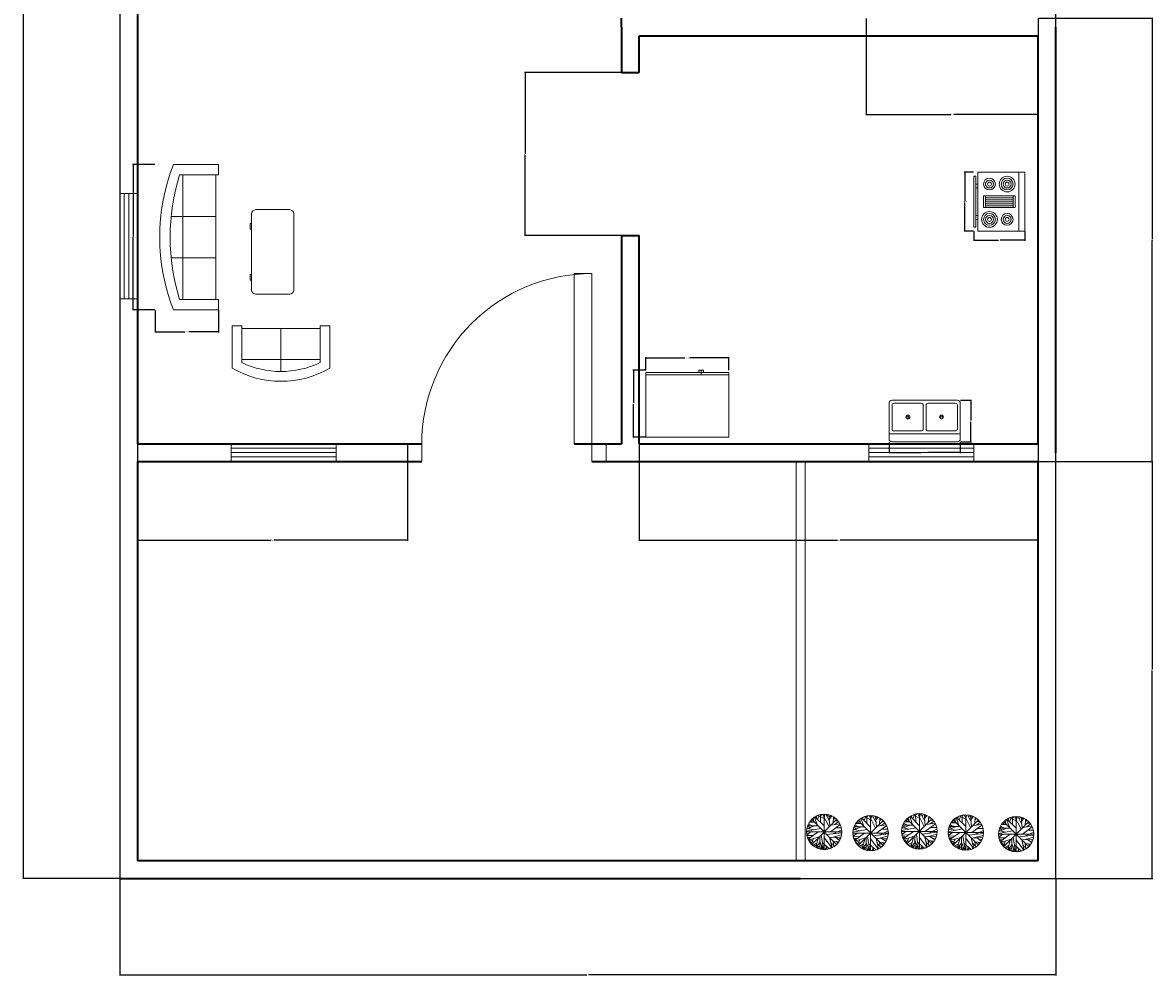
# Model space of a CAD drawing. Units: feet. Extents: x 2306 to 3052, y 829 to 1424.
# Tile 1 of 5: x 2306 to 2625, y 829 to 1098. Entities that reach past the tile are written whole.
import ezdxf

# ---------------------------------------------------------------- set-up
doc = ezdxf.new("R2010")
doc.units = ezdxf.units.FT
for name, color, linetype, lineweight in [('A-ANNO-DIMS', 2, 'Continuous', 18), ('A-DOOR', 3, 'Continuous', 18), ('A-EQPM', 9, 'Continuous', 18), ('A-FLOR-FIXT', 9, 'Continuous', 18), ('A-FLOR-OTLN', 7, 'Continuous', 25), ('A-FURN', 8, 'Continuous', 13), ('A-GLAZ', 4, 'Continuous', 18), ('A-WALL', 7, 'Continuous', 35), ('L-PLNT', 94, 'Continuous', 13)]:
    doc.layers.add(name, color=color, linetype=linetype, lineweight=lineweight)
doc.styles.get("Standard").update_dxf_attribs({"font": 'arial.ttf'})
doc.dimstyles.get("Standard").update_dxf_attribs({"dimtxt": 0.18, "dimasz": 0.18, "dimexe": 0.18, "dimexo": 0.0625, "dimgap": 0.09, "dimtad": 0, "dimtih": 1, "dimtoh": 1, "dimdec": 4, "dimzin": 0, "dimdsep": 46, "dimlunit": 4, "dimtxsty": 'Standard', "dimcen": 0.09, "dimadec": 0, "dimazin": 0, "dimtfac": 1, "dimtdec": 4, "dimtofl": 0, "dimtmove": 0, "dimatfit": 3, "dimfxl": 1, "dimtolj": 1, "dimtzin": 0, "dimarcsym": 0})

# ---------------------------------------------------------------- blocks, each defined once
blk = doc.blocks.new('Window - Wood Frame 36 in. Wide plan')
for p, q in [((0, 6), (0, 0)), ((0, 4.5), (36, 4.5)), ((36, 6), (36, 0)), ((0, 3), (36, 3)), ((0, 1.5), (36, 1.5))]:
    blk.add_line(p, q)
blk = doc.blocks.new('Sofa - Roundback 7 ft.')
for p, q in [((-36.000027, -34), (-36.000027, -11.4696)), ((-12.00002, -32.4421), (-12.00003, -6.5971)), ((11.99997, -32.4421), (11.99998, -6.5971)), ((35.99998, -34), (35.99998, -11.4696)), ((-35.999844, -13.3819), (35.9998, -13.3819)), ((-36.000027, -32.4421), (35.99998, -32.4421))]:
    blk.add_line(p, q)
for points in [[(-36.000027, -34), (-42.000027, -34), (-42.000027, -8)], [(41.99998, -8), (41.99998, -34), (35.99998, -34)]]:
    blk.add_lwpolyline(points)
for centre, radius, start, end in [((0, -114.25), 114.25, 68.43141, 111.5686), ((-0.00001, -127.1968), 121.1968, 72.72033, 107.2797)]:
    blk.add_arc(centre, radius, start, end)
blk = doc.blocks.new('Sofa - Roundback Loveseat 5 ft.')
for p, q in [((0, -32.44198), (0, -5.99998)), ((-24, -33.99998), (-24, -11.46958)), ((-23.9998, -13.38178), (23.99986, -13.38178)), ((24.00004, -33.99998), (24.00004, -11.46958)), ((-24, -32.44198), (24.00004, -32.44198))]:
    blk.add_line(p, q)
for points in [[(-24, -33.99998), (-30, -33.99998), (-30, -7.99998)], [(30.00004, -7.99998), (30.00004, -33.99998), (24.00004, -33.99998)]]:
    blk.add_lwpolyline(points)
for centre, radius, start, end in [((0, -60.24998), 60.24998, 60.13715, 119.8628), ((0, -61.38438), 55.38444, 64.32083, 115.6792)]:
    blk.add_arc(centre, radius, start, end)
blk = doc.blocks.new('Desk - 30 x 60 in.')
for p, q in [((-26.999995, 0), (26.999995, 0)), ((-29.999995, -27), (-29.999995, -3)), ((29.999995, -3), (29.999995, -27)), ((26.999995, -30), (-26.999995, -30)), ((-20.000005, -30), (-20.000005, -31)), ((-20.000005, -31), (-16.000005, -31)), ((-16.000005, -31), (-16.000005, -30)), ((15.999995, -31), (15.999995, -30)), ((19.999995, -31), (15.999995, -31)), ((19.999995, -30), (19.999995, -31))]:
    blk.add_line(p, q)
for centre, start, end in [((-26.499995, -3.5), 98.1301, 171.8699), ((26.499995, -3.5), 8.130102, 81.8699), ((-26.499995, -26.5), 188.1301, 261.8699), ((26.499995, -26.5), 278.1301, 351.8699)]:
    blk.add_arc(centre, 3.535534, start, end)
blk = doc.blocks.new('Range-Oven - 30 in top')
for p, q in [((0, -3), (30, -3)), ((12, -6), (18, -6)), ((13, -20), (13, -6)), ((14, -6), (14, -20)), ((15, -20), (15, -6)), ((16, -6), (16, -20)), ((17, -20), (17, -6)), ((18, -20), (12, -20)), ((6, -24), (6, -25)), ((8, -25), (8, -24)), ((22, -25), (22, -24)), ((24, -24), (24, -25))]:
    blk.add_line(p, q)
for points in [[(0, -24), (0, 0), (30, 0), (30, -24)], [(12, -21), (12, -5), (18, -5), (18, -21)], [(2, -26), (2, -25), (28, -25), (28, -26)]]:
    blk.add_lwpolyline(points, close=True)
for centre, radius in [((6, -9), 4), ((6, -9), 3), ((6, -9), 2), ((6, -9), 1), ((24, -9), 3), ((24, -9), 2), ((24, -9), 1), ((6, -18), 3), ((6, -18), 2), ((6, -18), 1), ((24, -18), 4), ((24, -18), 3), ((24, -18), 2), ((24, -18), 1)]:
    blk.add_circle(centre, radius)
blk = doc.blocks.new('Sink-double - 36 in top')
for p, q in [((-18, -4), (18, -4)), ((-0.75, -18.5), (-0.75, -6.5)), ((0.75, -6.5), (0.75, -18.5))]:
    blk.add_line(p, q)
for points in [[(-16.5, 0), (16.5, 0)], [(-18, -19.5), (-18, -1.5)], [(-15.5, -5.5), (-1.75, -5.5)], [(1.75, -5.5), (15.5, -5.5)], [(18, -1.5), (18, -19.5)], [(-16.5, -18.5), (-16.5, -6.5)], [(16.5, -6.5), (16.5, -18.5)], [(16.5, -21), (-16.5, -21)], [(-1.75, -19.5), (-15.5, -19.5)], [(15.5, -19.5), (1.75, -19.5)]]:
    blk.add_lwpolyline(points)
for centre, radius in [((-8.5, -12.5), 1), ((-8.5, -12.5), 0.5), ((8.5, -12.5), 1), ((8.5, -12.5), 0.5)]:
    blk.add_circle(centre, radius)
for centre, radius, start, end in [((-16.5, -1.5), 1.5, 90, 180), ((16.5, -1.5), 1.5, 0, 90), ((-15.5, -6.5), 1, 90, 180), ((-1.75, -6.5), 1, 0, 90), ((1.75, -6.5), 1, 90, 180), ((15.5, -6.5), 1, 0, 90), ((-16.5, -19.5), 1.5, 180, 270), ((-15.5, -18.5), 1, 180, 270), ((-1.75, -18.5), 1, 270, 0), ((1.75, -18.5), 1, 180, 270), ((15.5, -18.5), 1, 270, 0), ((16.5, -19.5), 1.5, 270, 0)]:
    blk.add_arc(centre, radius, start, end)
blk = doc.blocks.new('Refrigerator-2 door - 36 in top')
for p, q in [((0, -26.999999), (36, -26.999999)), ((11, -27.999999), (11, -28.999999)), ((11, -28.999999), (13, -28.999999)), ((12, -26.999999), (12, -28.999999)), ((13, -28.999999), (13, -27.999999))]:
    blk.add_line(p, q)
blk.add_lwpolyline([(0, -27.999999), (0, 0), (36, 0), (36, -27.999999)], close=True)
blk = doc.blocks.new('Tree - deciduous plan')
for p, q in [((-43.8768, 36.4326), (-44.405, 40.2696)), ((42, 42), (-42, -42)), ((42, -42), (-42, 42)), ((-40.1797, 44.558), (-36.4825, 43.2038)), ((-37.0107, 47.0408), (-35.25, 35.5298)), ((-32.6092, 50.4264), (-23.2782, 23.5674)), ((-31.2008, 51.1035), (-0.2149, 20.1818)), ((-26.4472, 46.5894), (-26.2712, 53.8116)), ((-22.0458, 42.0753), (-16.5881, 57.6486)), ((-21.1656, 55.8436), (-0.0388, 45.0094)), ((-12.5388, 54.9406), (-7.9613, 59.4546)), ((-12.3627, 32.1443), (-12.5388, 58.7776)), ((-5.3205, 59.6806), (16.5105, 16.7963)), ((2.426, 54.9406), (-1.4472, 59.9056)), ((0, 59.9996), (0, -60)), ((0.4894, 48.6208), (3.6584, 59.6806)), ((18.2711, 35.5298), (5.419, 59.6806)), ((9.8203, 51.5549), (12.8133, 58.5516)), ((19.6795, 19.5047), (16.3344, 57.6486)), ((17.0387, 51.1035), (23.2006, 55.1666)), ((17.7429, 43.6552), (25.4894, 54.2636)), ((31.6513, 50.8778), (30.2429, 30.5643)), ((31.1232, 42.5267), (35.8767, 48.1693)), ((-59.7219, 2.8025), (-12.0106, 12.0565)), ((-32.2571, 20.6333), (-59.1937, 9.348)), ((-58.6656, 12.7336), (-35.9543, 7.5424)), ((-57.081, 17.9248), (-47.0458, 14.7649)), ((-56.0247, 20.859), (-20.8134, 20.859)), ((-54.7923, 24.4702), (-47.75, 21.0847)), ((-54.6162, -24.7335), (-20.2853, 0.0941)), ((-53.2078, 27.4044), (-40.1797, 20.859)), ((-49.8627, 32.8214), (-32.7853, 32.8214)), ((-45.8134, 38.2383), (-40.5318, 33.0471)), ((54.3626, 25.3731), (20.9119, 0.3198)), ((23.3767, 23.3417), (53.3063, 27.4044)), ((29.3626, -6.6771), (59.4682, 7.091)), ((36.2288, 25.1474), (48.9049, 35.0784)), ((37.1091, 37.1098), (46.6161, 37.5612)), ((38.5175, 13.4107), (58.2359, 13.6364)), ((-60, 0), (60, 0)), ((-59.7219, -4.8714), (-54.2641, -6.6771)), ((-45.2853, -0.1316), (-59.0177, -10.0627)), ((-58.4895, -12.3197), (-36.4825, -11.6426)), ((-57.081, -18.4138), (-45.2853, -17.9624)), ((-52.6797, -18.188), (-55.4966, -22.0251)), ((-53.2078, -27.442), (-16.7641, -16.6081)), ((-38.9472, -29.0219), (-51.4472, -30.6018)), ((-47.2219, -19.3166), (-50.2148, -26.3135)), ((-46.5177, -30.1504), (-49.5106, -33.536)), ((-32.4331, -32.4075), (-48.1021, -35.5674)), ((-43.7008, -34.6645), (-46.6937, -37.373)), ((-35.9543, -22.4765), (-44.0529, -40.5329)), ((-24.6867, -37.8244), (-38.7712, -45.7241)), ((-19.9331, -20.2194), (-28.5599, -52.721)), ((-14.6515, -36.2445), (-27.6797, -52.9467)), ((-14.8275, -15.0282), (-14.6515, -57.6865)), ((-14.6515, -32.1818), (-3.912, -59.4922)), ((-10.074, -10.0627), (-2.5036, -59.7178)), ((-6.2008, -36.2445), (17.919, -57.0094)), ((-0.0388, -19.0909), (25.8415, -53.8495)), ((9.2922, -9.1598), (59.6443, -2.8401)), ((18.6232, -18.6394), (26.7218, -53.3981)), ((18.7992, -18.6394), (57.3556, -17.2853)), ((22.8485, -36.4702), (35.3485, -48.4326)), ((26.3697, -18.4138), (58.9401, -9.8369)), ((30.419, -30.1504), (32.3556, -50.0125)), ((31.4753, -31.279), (49.6091, -33.3103)), ((38.1654, -18.188), (52.426, -29.0219)), ((41.5105, -32.6332), (46.088, -38.0501)), ((45.9119, -24.0564), (55.595, -22.2508)), ((-26.2712, -43.9185), (-34.7219, -48.6583)), ((-14.6515, -47.3041), (-25.0388, -54.3009)), ((-21.5177, -45.4984), (-19.9331, -56.1065)), ((-8.4895, -47.5298), (-11.4825, -58.5893)), ((-6.3768, -52.721), (-9.3698, -58.815)), ((8.4119, -53.1724), (3.8344, -59.4922)), ((5.9471, -46.6269), (10.5246, -58.5893)), ((24.7852, -44.8213), (23.0246, -54.978))]:
    blk.add_line(p, q)
blk.add_circle((0, 0), 60)
blk = doc.blocks.new('DOOR-SWING-WIDE')
blk.add_lwpolyline([(52, 53), (52, 5), (56, 5), (56, 0), (52, 0), (52, 5), (47, 5), (47, 53), (48, 53), (52, 53, 0.414214), (4, 5)], format="xyb")
blk.add_lwpolyline([(4, 5), (4, 0), (0, 0), (0, 5)], close=True)
blk = doc.blocks.new('*D32')
at = {"layer": 'A-ANNO-DIMS', "color": 0, "lineweight": -2, "transparency": 16777216}
for p, q in [((2343.71, 1058.11), (2337.44, 1058.11)), ((2337.62, 1057.93), (2337.62, 1037.77)), ((2337.62, 1017.24), (2337.62, 1037.41)), ((2343.71, 1017.06), (2337.44, 1017.06))]:
    blk.add_line(p, q, dxfattribs=at)
at = {"layer": 'A-ANNO-DIMS', "color": 0, "transparency": 16777216}
for points in [[(2337.59, 1057.93), (2337.65, 1057.93), (2337.62, 1058.11)], [(2337.59, 1017.24), (2337.65, 1017.24), (2337.62, 1017.06)]]:
    blk.add_solid(points, dxfattribs=at)
at = {"layer": 'Defpoints', "color": 0, "transparency": 16777216}
for p in [(2337.62, 1058.11), (2343.77, 1058.11), (2343.77, 1017.06)]:
    blk.add_point(p, dxfattribs=at)
at = {"layer": 'A-ANNO-DIMS', "color": 0, "transparency": 16777216, "insert": (2337.62, 1037.59), "char_height": 0.18, "attachment_point": 5}
blk.add_mtext('\\A1;SOFA 41 TYP.', dxfattribs=at)
blk = doc.blocks.new('*D33')
at = {"layer": 'A-ANNO-DIMS', "color": 0, "lineweight": -2, "transparency": 16777216}
for p, q in [((2343.77, 1017), (2343.77, 1010.73)), ((2361.69, 1017), (2361.69, 1010.73)), ((2343.95, 1010.91), (2352.21, 1010.91)), ((2361.51, 1010.91), (2353.25, 1010.91))]:
    blk.add_line(p, q, dxfattribs=at)
at = {"layer": 'A-ANNO-DIMS', "color": 0, "transparency": 16777216}
for points in [[(2343.95, 1010.94), (2343.95, 1010.88), (2343.77, 1010.91)], [(2361.51, 1010.94), (2361.51, 1010.88), (2361.69, 1010.91)]]:
    blk.add_solid(points, dxfattribs=at)
at = {"layer": 'Defpoints', "color": 0, "transparency": 16777216}
for p in [(2343.77, 1017.06), (2361.69, 1017.06), (2343.77, 1010.91)]:
    blk.add_point(p, dxfattribs=at)
at = {"layer": 'A-ANNO-DIMS', "color": 0, "transparency": 16777216, "insert": (2352.73, 1010.91), "char_height": 0.18, "attachment_point": 5}
blk.add_mtext('\\A1;18 TYP.', dxfattribs=at)
blk = doc.blocks.new('*D40')
at = {"layer": 'A-ANNO-DIMS', "color": 0, "lineweight": -2, "transparency": 16777216}
for p, q in [((2574.57, 1055.88), (2571.96, 1055.88)), ((2572.14, 1055.7), (2572.14, 1047.76)), ((2572.14, 1039.45), (2572.14, 1047.39)), ((2574.57, 1039.27), (2571.96, 1039.27))]:
    blk.add_line(p, q, dxfattribs=at)
at = {"layer": 'A-ANNO-DIMS', "color": 0, "transparency": 16777216}
for points in [[(2572.11, 1055.7), (2572.17, 1055.7), (2572.14, 1055.88)], [(2572.11, 1039.45), (2572.17, 1039.45), (2572.14, 1039.27)]]:
    blk.add_solid(points, dxfattribs=at)
at = {"layer": 'Defpoints', "color": 0, "transparency": 16777216}
for p in [(2574.64, 1055.88), (2572.14, 1039.27), (2574.64, 1039.27)]:
    blk.add_point(p, dxfattribs=at)
at = {"layer": 'A-ANNO-DIMS', "color": 0, "transparency": 16777216, "insert": (2572.14, 1047.58), "char_height": 0.18, "attachment_point": 5}
blk.add_mtext('\\A1;RANGE 17', dxfattribs=at)
blk = doc.blocks.new('*D41')
at = {"layer": 'A-ANNO-DIMS', "color": 0, "lineweight": -2, "transparency": 16777216}
for p, q in [((2574.64, 1039.21), (2574.64, 1036.6)), ((2574.82, 1036.78), (2581.63, 1036.78)), ((2588.86, 1036.78), (2582.05, 1036.78)), ((2589.04, 1039.21), (2589.04, 1036.6))]:
    blk.add_line(p, q, dxfattribs=at)
at = {"layer": 'A-ANNO-DIMS', "color": 0, "transparency": 16777216}
for points in [[(2574.82, 1036.81), (2574.82, 1036.75), (2574.64, 1036.78)], [(2588.86, 1036.81), (2588.86, 1036.75), (2589.04, 1036.78)]]:
    blk.add_solid(points, dxfattribs=at)
at = {"layer": 'Defpoints', "color": 0, "transparency": 16777216}
for p in [(2574.64, 1039.27), (2589.04, 1039.27), (2589.04, 1036.78)]:
    blk.add_point(p, dxfattribs=at)
at = {"layer": 'A-ANNO-DIMS', "color": 0, "transparency": 16777216, "insert": (2581.84, 1036.78), "char_height": 0.18, "attachment_point": 5}
blk.add_mtext('\\A1;14', dxfattribs=at)
blk = doc.blocks.new('*D42')
at = {"layer": 'A-ANNO-DIMS', "color": 0, "lineweight": -2, "transparency": 16777216}
for p, q in [((2550.75, 979.83), (2550.75, 976.7)), ((2570.84, 979.83), (2570.84, 976.7)), ((2550.93, 976.88), (2559.7, 976.88)), ((2570.66, 976.88), (2561.89, 976.88))]:
    blk.add_line(p, q, dxfattribs=at)
at = {"layer": 'A-ANNO-DIMS', "color": 0, "transparency": 16777216}
for points in [[(2550.93, 976.91), (2550.93, 976.85), (2550.75, 976.88)], [(2570.66, 976.91), (2570.66, 976.85), (2570.84, 976.88)]]:
    blk.add_solid(points, dxfattribs=at)
at = {"layer": 'Defpoints', "color": 0, "transparency": 16777216}
for p in [(2550.75, 979.89), (2570.84, 979.89), (2550.75, 976.88)]:
    blk.add_point(p, dxfattribs=at)
at = {"layer": 'A-ANNO-DIMS', "color": 0, "transparency": 16777216, "insert": (2560.79, 976.88), "char_height": 0.18, "attachment_point": 5}
blk.add_mtext('\\A1;DOUBLE SINK 20', dxfattribs=at)
blk = doc.blocks.new('*D43')
at = {"layer": 'A-ANNO-DIMS', "color": 0, "lineweight": -2, "transparency": 16777216}
for p, q in [((2570.9, 991.61), (2574.03, 991.61)), ((2573.85, 991.43), (2573.85, 985.93)), ((2573.85, 980.07), (2573.85, 985.57)), ((2570.9, 979.89), (2574.03, 979.89))]:
    blk.add_line(p, q, dxfattribs=at)
at = {"layer": 'A-ANNO-DIMS', "color": 0, "transparency": 16777216}
for points in [[(2573.82, 991.43), (2573.88, 991.43), (2573.85, 991.61)], [(2573.82, 980.07), (2573.88, 980.07), (2573.85, 979.89)]]:
    blk.add_solid(points, dxfattribs=at)
at = {"layer": 'Defpoints', "color": 0, "transparency": 16777216}
for p in [(2570.84, 991.61), (2570.84, 979.89), (2573.85, 979.89)]:
    blk.add_point(p, dxfattribs=at)
at = {"layer": 'A-ANNO-DIMS', "color": 0, "transparency": 16777216, "insert": (2573.85, 985.75), "char_height": 0.18, "attachment_point": 5}
blk.add_mtext('\\A1;12', dxfattribs=at)
blk = doc.blocks.new('*D44')
at = {"layer": 'A-ANNO-DIMS', "color": 0, "lineweight": -2, "transparency": 16777216}
for p, q in [((2482.2, 1000.12), (2482.2, 1003.74)), ((2482.38, 1003.56), (2493.15, 1003.56)), ((2505.37, 1003.56), (2494.6, 1003.56)), ((2505.55, 1000.12), (2505.55, 1003.74))]:
    blk.add_line(p, q, dxfattribs=at)
at = {"layer": 'A-ANNO-DIMS', "color": 0, "transparency": 16777216}
for points in [[(2482.38, 1003.59), (2482.38, 1003.53), (2482.2, 1003.56)], [(2505.37, 1003.59), (2505.37, 1003.53), (2505.55, 1003.56)]]:
    blk.add_solid(points, dxfattribs=at)
at = {"layer": 'Defpoints', "color": 0, "transparency": 16777216}
for p in [(2482.2, 1003.56), (2482.2, 1000.06), (2505.55, 1000.06)]:
    blk.add_point(p, dxfattribs=at)
at = {"layer": 'A-ANNO-DIMS', "color": 0, "transparency": 16777216, "insert": (2493.87, 1003.56), "char_height": 0.18, "attachment_point": 5}
blk.add_mtext('\\A1;FRIDGE 23', dxfattribs=at)
blk = doc.blocks.new('*D45')
at = {"layer": 'A-ANNO-DIMS', "color": 0, "lineweight": -2, "transparency": 16777216}
for p, q in [((2482.13, 1000.06), (2478.51, 1000.06)), ((2478.69, 999.88), (2478.69, 990.84)), ((2478.69, 981.43), (2478.69, 990.48)), ((2482.13, 981.25), (2478.51, 981.25))]:
    blk.add_line(p, q, dxfattribs=at)
at = {"layer": 'A-ANNO-DIMS', "color": 0, "transparency": 16777216}
for points in [[(2478.66, 999.88), (2478.72, 999.88), (2478.69, 1000.06)], [(2478.66, 981.43), (2478.72, 981.43), (2478.69, 981.25)]]:
    blk.add_solid(points, dxfattribs=at)
at = {"layer": 'Defpoints', "color": 0, "transparency": 16777216}
for p in [(2482.2, 1000.06), (2478.69, 981.25), (2482.2, 981.25)]:
    blk.add_point(p, dxfattribs=at)
at = {"layer": 'A-ANNO-DIMS', "color": 0, "transparency": 16777216, "insert": (2478.69, 990.66), "char_height": 0.18, "attachment_point": 5}
blk.add_mtext('\\A1;19', dxfattribs=at)
blk = doc.blocks.new('*D46')
at = {"layer": 'A-ANNO-DIMS', "color": 0, "lineweight": -2, "transparency": 16777216}
for p, q in [((2333.8, 856.76), (2333.8, 829.47)), ((2597.8, 856.76), (2597.8, 829.47)), ((2333.98, 829.65), (2465.51, 829.65)), ((2597.62, 829.65), (2466.09, 829.65))]:
    blk.add_line(p, q, dxfattribs=at)
at = {"layer": 'A-ANNO-DIMS', "color": 0, "transparency": 16777216}
for points in [[(2333.98, 829.68), (2333.98, 829.62), (2333.8, 829.65)], [(2597.62, 829.68), (2597.62, 829.62), (2597.8, 829.65)]]:
    blk.add_solid(points, dxfattribs=at)
at = {"layer": 'Defpoints', "color": 0, "transparency": 16777216}
for p in [(2333.8, 856.83), (2597.8, 856.83), (2597.8, 829.65)]:
    blk.add_point(p, dxfattribs=at)
at = {"layer": 'A-ANNO-DIMS', "color": 0, "transparency": 16777216, "insert": (2465.8, 829.65), "char_height": 0.18, "attachment_point": 5}
blk.add_mtext('\\A1;264', dxfattribs=at)
blk = doc.blocks.new('*D47')
at = {"layer": 'A-ANNO-DIMS', "color": 0, "lineweight": -2, "transparency": 16777216}
for p, q in [((2333.74, 1396.83), (2306.45, 1396.83)), ((2306.63, 1396.65), (2306.63, 1127.01)), ((2306.63, 857.01), (2306.63, 1126.65)), ((2333.74, 856.83), (2306.45, 856.83))]:
    blk.add_line(p, q, dxfattribs=at)
at = {"layer": 'A-ANNO-DIMS', "color": 0, "transparency": 16777216}
for points in [[(2306.6, 1396.65), (2306.66, 1396.65), (2306.63, 1396.83)], [(2306.6, 857.01), (2306.66, 857.01), (2306.63, 856.83)]]:
    blk.add_solid(points, dxfattribs=at)
at = {"layer": 'Defpoints', "color": 0, "transparency": 16777216}
for p in [(2306.63, 1396.83), (2333.8, 1396.83), (2333.8, 856.83)]:
    blk.add_point(p, dxfattribs=at)
at = {"layer": 'A-ANNO-DIMS', "color": 0, "transparency": 16777216, "insert": (2306.63, 1126.83), "char_height": 0.18, "attachment_point": 5}
blk.add_mtext('\\A1;540', dxfattribs=at)
blk = doc.blocks.new('*D48')
at = {"layer": 'A-ANNO-DIMS', "color": 0, "lineweight": -2, "transparency": 16777216}
for p, q in [((2592.87, 974.33), (2625.16, 974.33)), ((2624.98, 974.15), (2624.98, 915.76)), ((2624.98, 857.01), (2624.98, 915.4)), ((2597.87, 856.83), (2625.16, 856.83))]:
    blk.add_line(p, q, dxfattribs=at)
at = {"layer": 'A-ANNO-DIMS', "color": 0, "transparency": 16777216}
for points in [[(2624.95, 974.15), (2625.01, 974.15), (2624.98, 974.33)], [(2624.95, 857.01), (2625.01, 857.01), (2624.98, 856.83)]]:
    blk.add_solid(points, dxfattribs=at)
at = {"layer": 'Defpoints', "color": 0, "transparency": 16777216}
for p in [(2592.8, 974.33), (2624.98, 974.33), (2597.8, 856.83)]:
    blk.add_point(p, dxfattribs=at)
at = {"layer": 'A-ANNO-DIMS', "color": 0, "transparency": 16777216, "insert": (2624.98, 915.58), "char_height": 0.18, "attachment_point": 5}
blk.add_mtext('\\A1;117.5', dxfattribs=at)
blk = doc.blocks.new('*D49')
at = {"layer": 'A-ANNO-DIMS', "color": 0, "lineweight": -2, "transparency": 16777216}
for p, q in [((2592.87, 1099.33), (2625.16, 1099.33)), ((2624.98, 1099.15), (2624.98, 1037.01)), ((2624.98, 974.51), (2624.98, 1036.65)), ((2592.87, 974.33), (2625.16, 974.33))]:
    blk.add_line(p, q, dxfattribs=at)
at = {"layer": 'A-ANNO-DIMS', "color": 0, "transparency": 16777216}
for points in [[(2624.95, 1099.15), (2625.01, 1099.15), (2624.98, 1099.33)], [(2624.95, 974.51), (2625.01, 974.51), (2624.98, 974.33)]]:
    blk.add_solid(points, dxfattribs=at)
at = {"layer": 'Defpoints', "color": 0, "transparency": 16777216}
for p in [(2592.8, 1099.33), (2624.98, 1099.33), (2592.8, 974.33)]:
    blk.add_point(p, dxfattribs=at)
at = {"layer": 'A-ANNO-DIMS', "color": 0, "transparency": 16777216, "insert": (2624.98, 1036.83), "char_height": 0.18, "attachment_point": 5}
blk.add_mtext('\\A1;125', dxfattribs=at)
blk = doc.blocks.new('*D57')
at = {"layer": 'A-ANNO-DIMS', "color": 0, "lineweight": -2, "transparency": 16777216}
for p, q in [((2480.3, 979.26), (2480.3, 951.97)), ((2592.8, 979.26), (2592.8, 951.97)), ((2480.48, 952.15), (2536.17, 952.15)), ((2592.62, 952.15), (2536.94, 952.15))]:
    blk.add_line(p, q, dxfattribs=at)
at = {"layer": 'A-ANNO-DIMS', "color": 0, "transparency": 16777216}
for points in [[(2480.48, 952.18), (2480.48, 952.12), (2480.3, 952.15)], [(2592.62, 952.18), (2592.62, 952.12), (2592.8, 952.15)]]:
    blk.add_solid(points, dxfattribs=at)
at = {"layer": 'Defpoints', "color": 0, "transparency": 16777216}
for p in [(2480.3, 979.33), (2592.8, 979.33), (2480.3, 952.15)]:
    blk.add_point(p, dxfattribs=at)
at = {"layer": 'A-ANNO-DIMS', "color": 0, "transparency": 16777216, "insert": (2536.55, 952.15), "char_height": 0.18, "attachment_point": 5}
blk.add_mtext('\\A1;112.5', dxfattribs=at)
blk = doc.blocks.new('*D58')
at = {"layer": 'A-ANNO-DIMS', "color": 0, "lineweight": -2, "transparency": 16777216}
for p, q in [((2338.8, 979.26), (2338.8, 951.97)), ((2414.97, 979.26), (2414.97, 951.97)), ((2338.98, 952.15), (2376.5, 952.15)), ((2414.79, 952.15), (2377.28, 952.15))]:
    blk.add_line(p, q, dxfattribs=at)
at = {"layer": 'A-ANNO-DIMS', "color": 0, "transparency": 16777216}
for points in [[(2338.98, 952.18), (2338.98, 952.12), (2338.8, 952.15)], [(2414.79, 952.18), (2414.79, 952.12), (2414.97, 952.15)]]:
    blk.add_solid(points, dxfattribs=at)
at = {"layer": 'Defpoints', "color": 0, "transparency": 16777216}
for p in [(2338.8, 979.33), (2414.97, 979.33), (2338.8, 952.15)]:
    blk.add_point(p, dxfattribs=at)
at = {"layer": 'A-ANNO-DIMS', "color": 0, "transparency": 16777216, "insert": (2376.89, 952.15), "char_height": 0.18, "attachment_point": 5}
blk.add_mtext('\\A1;76.17', dxfattribs=at)
blk = doc.blocks.new('*D60')
at = {"layer": 'A-ANNO-DIMS', "color": 0, "lineweight": -2, "transparency": 16777216}
for p, q in [((2475.24, 1083.97), (2447.95, 1083.97)), ((2448.13, 1083.79), (2448.13, 1061.21)), ((2448.13, 1038.26), (2448.13, 1060.84)), ((2475.24, 1038.08), (2447.95, 1038.08))]:
    blk.add_line(p, q, dxfattribs=at)
at = {"layer": 'A-ANNO-DIMS', "color": 0, "transparency": 16777216}
for points in [[(2448.1, 1083.79), (2448.16, 1083.79), (2448.13, 1083.97)], [(2448.1, 1038.26), (2448.16, 1038.26), (2448.13, 1038.08)]]:
    blk.add_solid(points, dxfattribs=at)
at = {"layer": 'Defpoints', "color": 0, "transparency": 16777216}
for p in [(2448.13, 1083.97), (2475.3, 1083.97), (2475.3, 1038.08)]:
    blk.add_point(p, dxfattribs=at)
at = {"layer": 'A-ANNO-DIMS', "color": 0, "transparency": 16777216, "insert": (2448.13, 1061.02), "char_height": 0.18, "attachment_point": 5}
blk.add_mtext('\\A1;45.89', dxfattribs=at)
blk = doc.blocks.new('*D61')
at = {"layer": 'A-ANNO-DIMS', "color": 0, "lineweight": -2, "transparency": 16777216}
for p, q in [((2544.34, 1099.26), (2544.34, 1071.97)), ((2592.8, 1099.26), (2592.8, 1071.97)), ((2544.52, 1072.15), (2568.17, 1072.15)), ((2592.62, 1072.15), (2568.97, 1072.15))]:
    blk.add_line(p, q, dxfattribs=at)
at = {"layer": 'A-ANNO-DIMS', "color": 0, "transparency": 16777216}
for points in [[(2544.52, 1072.18), (2544.52, 1072.12), (2544.34, 1072.15)], [(2592.62, 1072.18), (2592.62, 1072.12), (2592.8, 1072.15)]]:
    blk.add_solid(points, dxfattribs=at)
at = {"layer": 'Defpoints', "color": 0, "transparency": 16777216}
for p in [(2544.34, 1099.33), (2592.8, 1099.33), (2544.34, 1072.15)]:
    blk.add_point(p, dxfattribs=at)
at = {"layer": 'A-ANNO-DIMS', "color": 0, "transparency": 16777216, "insert": (2568.57, 1072.15), "char_height": 0.18, "attachment_point": 5}
blk.add_mtext('\\A1;48.47', dxfattribs=at)

msp = doc.modelspace()

# ---------------------------------------------------------------- linework, layer by layer
at = {"layer": 'A-FLOR-OTLN'}
for p, q in [((2333.803, 1396.827), (2333.803, 856.827)), ((2597.803, 856.827), (2597.803, 1396.827)), ((2333.803, 856.827), (2597.803, 856.827))]:
    msp.add_line(p, q, dxfattribs=at)
at = {"layer": 'A-WALL'}
for p, q in [((2338.803, 1250.327), (2338.803, 979.327)), ((2475.303, 1096.827), (2475.303, 1099.327)), ((2475.303, 1096.827), (2475.303, 1083.971)), ((2480.303, 1094.327), (2592.803, 1094.327)), ((2480.303, 1083.971), (2480.303, 1094.327)), ((2592.803, 979.327), (2592.803, 1094.327)), ((2597.803, 976.827), (2597.803, 1096.827)), ((2475.303, 1083.971), (2480.303, 1083.971)), ((2475.303, 1038.077), (2480.303, 1038.077)), ((2475.303, 1038.077), (2475.303, 979.327)), ((2480.303, 979.327), (2480.303, 1038.077)), ((2338.803, 979.327), (2418.974, 979.327)), ((2461.974, 979.327), (2475.303, 979.327)), ((2480.303, 979.327), (2501.803, 979.327)), ((2501.803, 979.327), (2592.803, 979.327)), ((2338.803, 974.327), (2418.974, 974.327)), ((2338.803, 974.327), (2338.803, 861.827)), ((2466.974, 974.327), (2501.803, 974.327)), ((2501.803, 974.327), (2592.803, 974.327)), ((2523.303, 974.327), (2525.803, 974.327)), ((2592.803, 861.827), (2592.803, 974.327)), ((2338.803, 861.827), (2592.803, 861.827)), ((2338.803, 861.827), (2525.803, 861.827)), ((2333.803, 856.827), (2525.803, 856.827))]:
    msp.add_line(p, q, dxfattribs=at)
at = {"layer": 'L-PLNT'}
for p, q in [((2524.553, 974.327), (2524.553, 861.827)), ((2524.553, 974.327), (2527.053, 974.327)), ((2527.053, 861.827), (2527.053, 974.327))]:
    msp.add_line(p, q, dxfattribs=at)

# ---------------------------------------------------------------- block references
at = {"layer": 'A-DOOR'}
msp.add_blockref('DOOR-SWING-WIDE', (2414.974, 974.327), dxfattribs=at)
at = {"layer": 'A-EQPM'}
for name, p, xscale, yscale, zscale, rotation in [('Range-Oven - 30 in top', (2589.035, 1055.884), 0.5538035962556707, 0.5538035962556707, 0.5538035962556707, 270), ('Refrigerator-2 door - 36 in top', (2505.547, 981.252), 0.6485986588828088, 0.6485986588828088, 0.6485986588828088, 180)]:
    msp.add_blockref(name, p, dxfattribs=dict(at, xscale=xscale, yscale=yscale, zscale=zscale, rotation=rotation))
at = {"layer": 'A-FLOR-FIXT', "xscale": 0.5580233951230867, "yscale": 0.5580233951230867, "zscale": 0.5580233951230867, "rotation": 180}
msp.add_blockref('Sink-double - 36 in top', (2560.794, 979.895), dxfattribs=at)
at = {"layer": 'A-FURN'}
for name, p, xscale, yscale, zscale, rotation in [('Sofa - Roundback 7 ft.', (2345.076, 1037.589), 0.4886678051459193, 0.4886678051459193, 0.4886678051459193, 90), ('Desk - 30 x 60 in.', (2382.902, 1033.44), 0.3981448877142051, 0.3981448877142051, 0.3981448877142051, 270), ('Sofa - Roundback Loveseat 5 ft.', (2379.267, 996.965), 0.4591894755531339, 0.4591894755531339, 0.4591894755531339, 180)]:
    msp.add_blockref(name, p, dxfattribs=dict(at, xscale=xscale, yscale=yscale, zscale=zscale, rotation=rotation))
at = {"layer": 'A-GLAZ', "xscale": 0.82338841385576, "yscale": 0.82338841385576, "zscale": 0.82338841385576, "rotation": 90}
msp.add_blockref('Window - Wood Frame 36 in. Wide plan', (2338.803, 1020.247), dxfattribs=at)
at = {"layer": 'A-GLAZ', "xscale": 0.82338841385576, "yscale": 0.82338841385576, "zscale": 0.82338841385576}
for p in [(2365.2, 974.387), (2545.006, 974.387)]:
    msp.add_blockref('Window - Wood Frame 36 in. Wide plan', p, dxfattribs=at)
at = {"layer": 'L-PLNT', "xscale": 0.0833333333333333, "yscale": 0.0833333333333333, "zscale": 0.0833333333333333}
for p in [(2532.448, 869.911), (2545.547, 869.592), (2559.286, 870.071), (2572.385, 869.751), (2586.605, 869.261)]:
    msp.add_blockref('Tree - deciduous plan', p, dxfattribs=at)

# ---------------------------------------------------------------- dimensions: what is measured, and where the dimension line sits
at = {"layer": 'A-ANNO-DIMS'}
for base, p1, p2, angle, override, picture, middle in [((2306.628, 1396.827), (2333.803, 856.827), (2333.803, 1396.827), 90, {"dimdec": 0, "dimlfac": 1, "dimrnd": 0, "dimzin": 0, "dimdsep": 46, "dimlunit": 2}, '*D47', (2306.628, 1126.827)), ((2544.336, 1072.152), (2592.803, 1099.327), (2544.336, 1099.327), 180, {"dimdec": 2, "dimlfac": 1, "dimrnd": 0, "dimzin": 0, "dimdsep": 46, "dimlunit": 2}, '*D61', (2568.57, 1072.152)), ((2624.978, 1099.327), (2592.803, 974.327), (2592.803, 1099.327), 90, {"dimdec": 0, "dimlfac": 1, "dimrnd": 0, "dimzin": 0, "dimdsep": 46, "dimlunit": 2}, '*D49', (2624.978, 1036.827)), ((2448.128, 1083.971), (2475.303, 1038.077), (2475.303, 1083.971), 90, {"dimdec": 2, "dimlfac": 1, "dimrnd": 0, "dimzin": 0, "dimdsep": 46, "dimlunit": 2}, '*D60', (2448.128, 1061.024)), ((2478.695, 981.252), (2482.197, 1000.062), (2482.197, 981.252), 270, {"dimdec": 0, "dimlfac": 1, "dimrnd": 0, "dimzin": 0, "dimdsep": 46, "dimlunit": 2}, '*D45', (2478.695, 990.657)), ((2573.852, 979.895), (2570.838, 991.613), (2570.838, 979.895), 270, {"dimdec": 0, "dimlfac": 1, "dimrnd": 0, "dimzin": 0, "dimdsep": 46, "dimlunit": 2}, '*D43', (2573.852, 985.754)), ((2338.803, 952.152), (2414.974, 979.327), (2338.803, 979.327), 180, {"dimdec": 2, "dimlfac": 1, "dimrnd": 0, "dimzin": 0, "dimdsep": 46, "dimlunit": 2}, '*D58', (2376.889, 952.152)), ((2480.303, 952.152), (2592.803, 979.327), (2480.303, 979.327), 180, {"dimdec": 1, "dimlfac": 1, "dimrnd": 0, "dimzin": 0, "dimdsep": 46, "dimlunit": 2}, '*D57', (2536.553, 952.152)), ((2624.978, 974.327), (2597.803, 856.827), (2592.803, 974.327), 90, {"dimdec": 1, "dimlfac": 1, "dimrnd": 0, "dimzin": 0, "dimdsep": 46, "dimlunit": 2}, '*D48', (2624.978, 915.577))]:
    dim = msp.add_linear_dim(base=base, p1=p1, p2=p2, angle=angle, dimstyle='Standard', override=override, dxfattribs=at)
    dim.commit()
    dim.dimension.update_dxf_attribs({"geometry": picture, "text_midpoint": middle})
for base, p1, p2, angle, text, picture, middle in [((2337.616, 1058.113), (2343.773, 1017.065), (2343.773, 1058.113), 90, 'SOFA <> TYP.', '*D32', (2337.616, 1037.589)), ((2572.144, 1039.27), (2574.636, 1055.884), (2574.636, 1039.27), 270, 'RANGE <>', '*D40', (2572.144, 1047.577)), ((2343.773, 1010.907), (2361.691, 1017.065), (2343.773, 1017.065), 180, '<> TYP.', '*D33', (2352.732, 1010.907)), ((2482.197, 1003.564), (2505.547, 1000.062), (2482.197, 1000.062), 180, 'FRIDGE <>', '*D44', (2493.872, 1003.564)), ((2550.749, 976.881), (2570.838, 979.895), (2550.749, 979.895), 180, 'DOUBLE SINK <>', '*D42', (2560.794, 976.881))]:
    dim = msp.add_linear_dim(base=base, p1=p1, p2=p2, angle=angle, text=text, dimstyle='Standard', override={"dimdec": 0, "dimlfac": 1, "dimrnd": 0, "dimzin": 0, "dimdsep": 46, "dimlunit": 2}, dxfattribs=at)
    dim.commit()
    dim.dimension.update_dxf_attribs({"geometry": picture, "text_midpoint": middle})
for base, p1, p2, picture, middle in [((2589.035, 1036.778), (2574.636, 1039.27), (2589.035, 1039.27), '*D41', (2581.836, 1036.778)), ((2597.803, 829.652), (2333.803, 856.827), (2597.803, 856.827), '*D46', (2465.803, 829.652))]:
    dim = msp.add_linear_dim(base=base, p1=p1, p2=p2, dimstyle='Standard', override={"dimdec": 0, "dimlfac": 1, "dimrnd": 0, "dimzin": 0, "dimdsep": 46, "dimlunit": 2}, dxfattribs=at)
    dim.commit()
    dim.dimension.update_dxf_attribs({"geometry": picture, "text_midpoint": middle})

doc.saveas('drawing.dxf')
